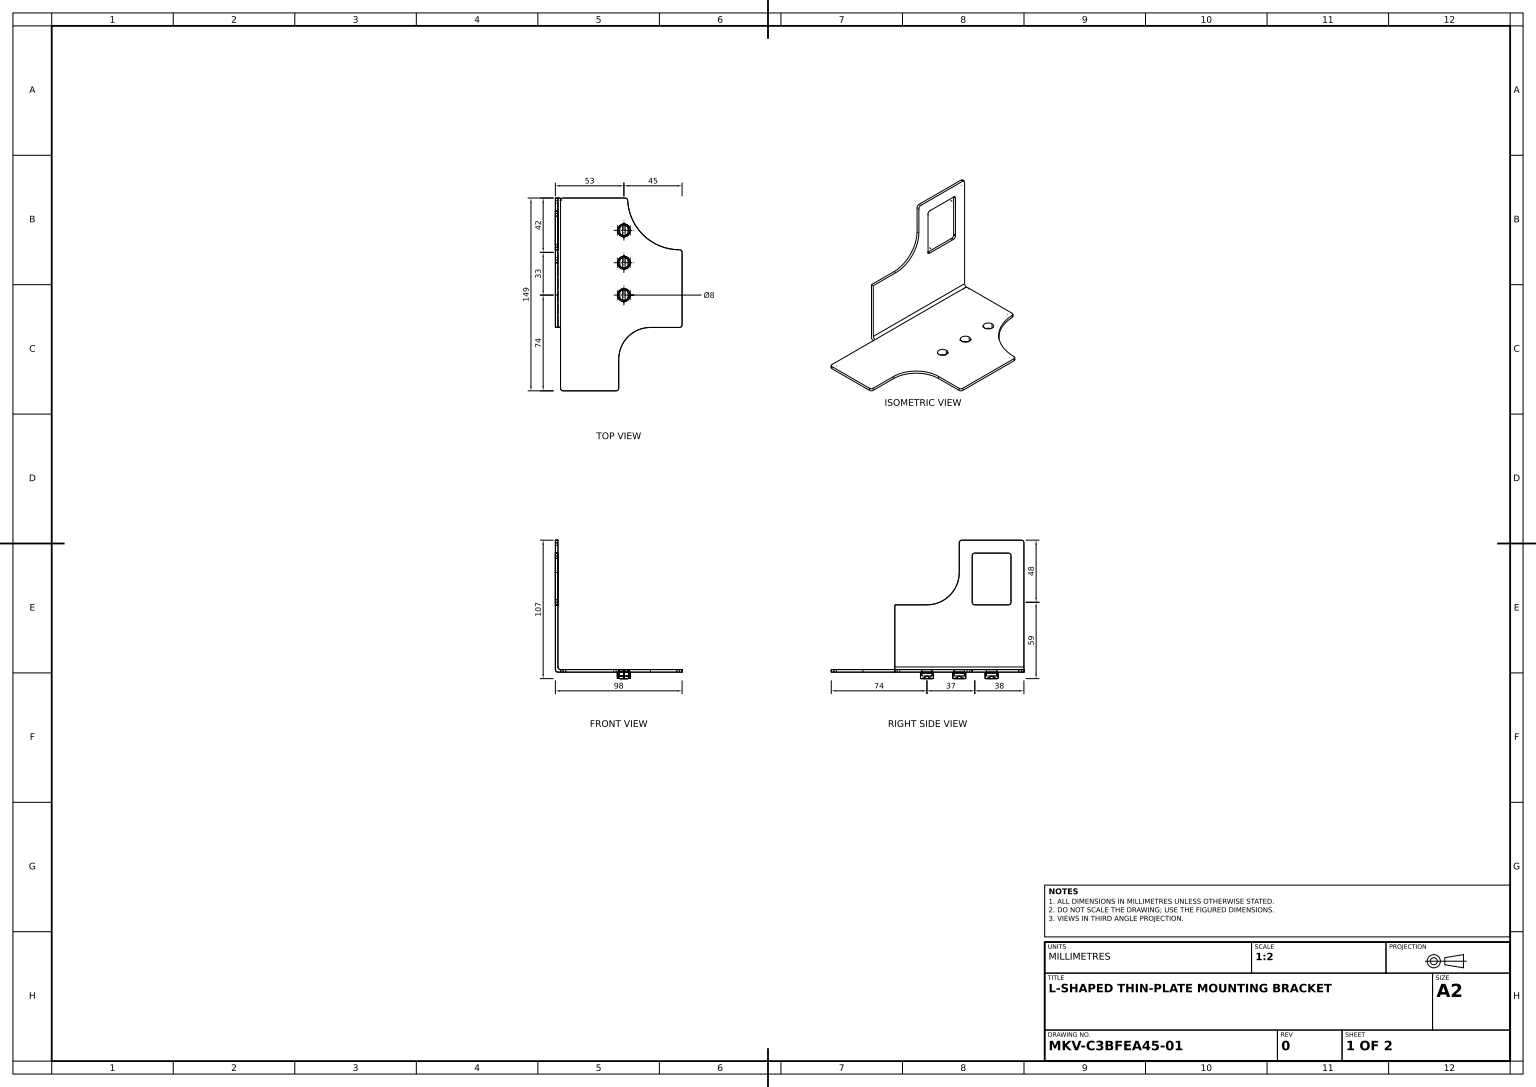
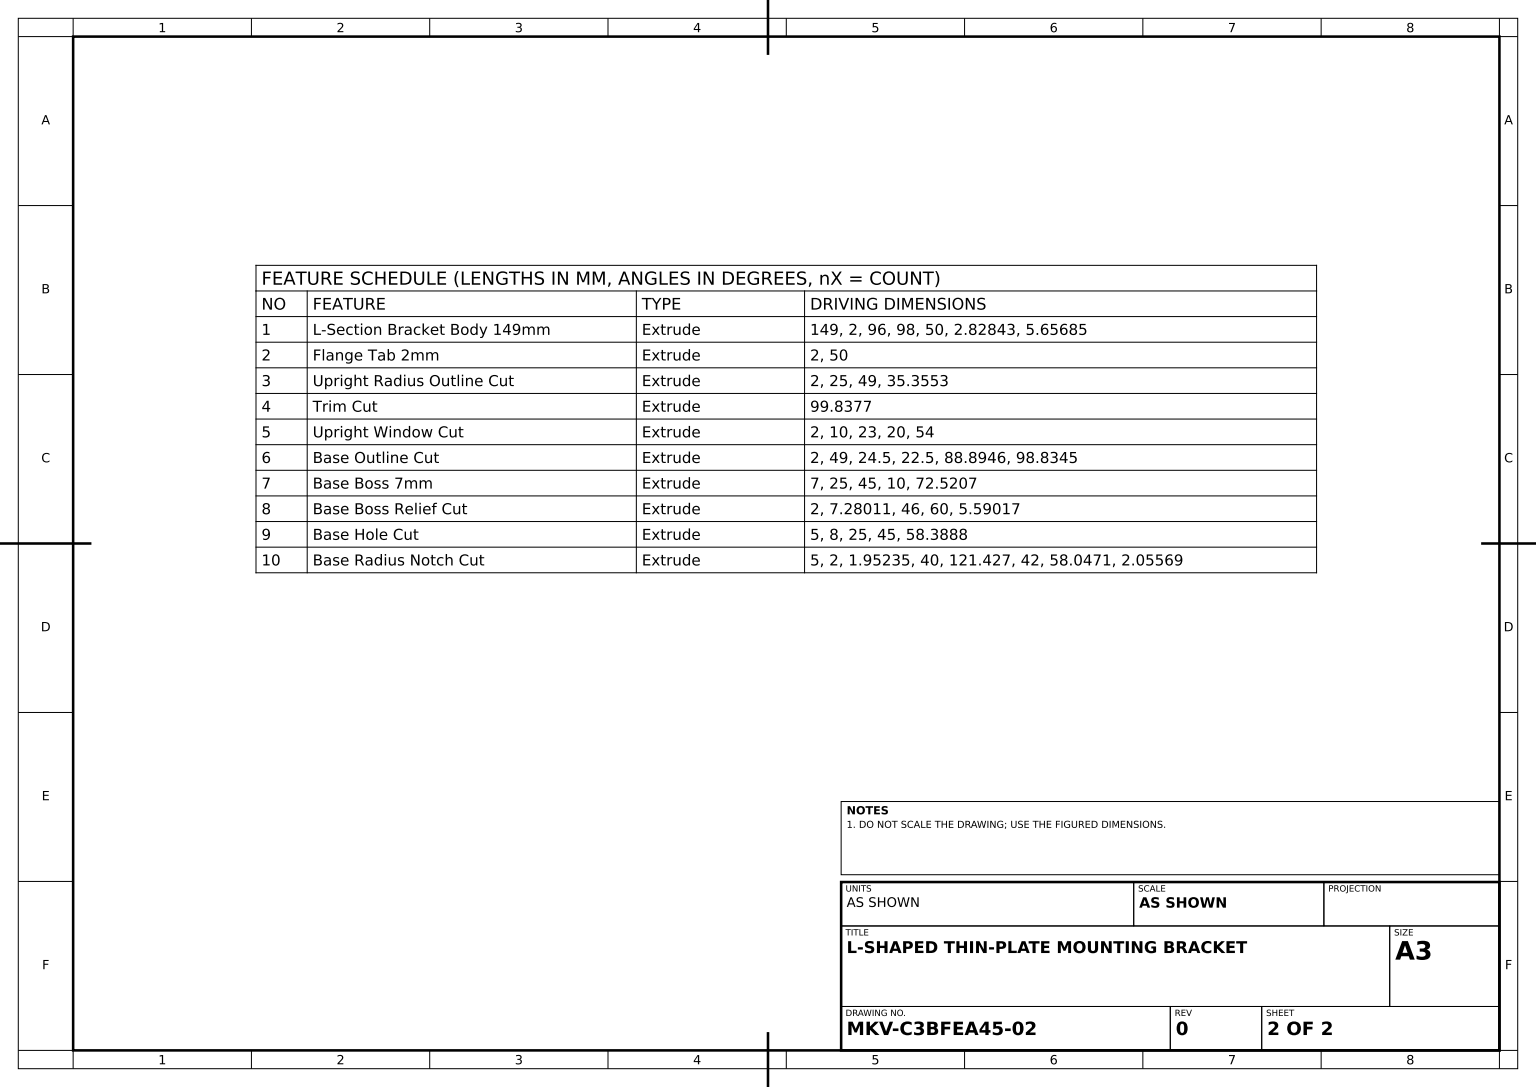
SolidWorks part; units mm, degrees
material "Plain Carbon Steel"
ref_plane "Front Plane" through (0, 0, 0) normal (0, 0, 1) x (1, 0, 0)
ref_plane "Top Plane" through (0, 0, 0) normal (0, 1, 0) x (1, 0, 0)
ref_plane "Right Plane" through (0, 0, 0) normal (1, 0, 0) x (0, 0, -1)
sketch "L-Section Profile Sketch" plane through (0, 0, 0) normal (0, 0, 1) x (1, 0, 0)
  line L0 (2, 0) -> (98, 0)
  line L4 (0, 2) -> (0, 52)
  line L5 (0, 52) -> (2, 52)
  line L6 (2, 52) -> (2, 4)
  line L7 (4, 2) -> (98, 2)
  line L8 (98, 2) -> (98, 0)
  arc A0 (2, 4) -> (4, 2) centre (4, 4) ccw
  arc A2 (0, 2) -> (2, 0) centre (2, 2) ccw
  dimension "D2" = 2
  dimension "D1" = 2
  dimension "D3" = 96
  dimension "D4" = 98
  dimension "D5" = 50
  dimension "D6" = 2
  dimension "D7" = 2
  dimension "D8" = 2.8284
  dimension "D9" = 5.6569
extrude "L-Section Bracket Body 149mm" add sketch "L-Section Profile Sketch" along normal mid plane 149
sketch "Flange Tab Sketch" plane through (2, 0, 0) normal (1, 0, 0) x (0, 0, -1)
  line L0 (74.5, 52) -> (74.5, 102)
  line L1 (74.5, 102) -> (-74.5, 102)
  line L2 (-74.5, 102) -> (-74.5, 52)
  line L3 (-74.5, 52) -> (74.5, 52)
  line L5 (-74.5, 52) -> (74.5, 52) construction
  dimension "D1" = 50
extrude "Flange Tab 2mm" add sketch "Flange Tab Sketch" against normal blind 2
sketch "Upright Radius Outline Sketch" plane through (2, 0, 0) normal (1, 0, 0) x (0, 0, -1)
  line L0 (24.5, 102) -> (-74.5, 102)
  line L1 (-74.5, 102) -> (-74.5, 4)
  line L2 (74.5, 102) -> (-74.5, 102) construction
  line L3 (-74.5, 4) -> (-25.5, 4)
  line L4 (-74.5, 4) -> (74.5, 4) construction
  line L5 (-25.5, 4) -> (-25.5, 52)
  line L6 (-25.5, 52) -> (-0.5, 52)
  line L7 (24.5, 77) -> (24.5, 102)
  arc A0 (-0.5, 52) -> (24.5, 77) centre (-0.5, 77) ccw
  dimension "D1" = 25
  dimension "D2" = 25
  dimension "D3" = 49
  dimension "D4" = 35.3553
extrude "Upright Radius Outline Cut" cut sketch "Upright Radius Outline Sketch" against normal blind 2
sketch "Trim Cut Sketch" plane through (0, 2, 0) normal (0, 1, 0) x (1, 0, 0)
  line L0 (0, -25.3377) -> (4, -25.3377)
  line L1 (4, -74.5) -> (4, 74.5) construction
  line L2 (4, -25.3377) -> (4, -74.5)
  line L3 (4, -74.5) -> (0, -74.5)
  line L4 (0, -74.5) -> (0, -25.3377)
  line L5 (98, 74.5) -> (4, 74.5) construction
  dimension "D1" = 99.8377
extrude "Trim Cut" cut sketch "Trim Cut Sketch" along normal through all both and the other way through all
sketch "Upright Window Sketch" plane through (2, 0, 0) normal (1, 0, 0) x (0, 0, -1)
  line L0 (74.5, 102) -> (72.5, 102)
  line L2 (-25.3377, 4) -> (74.5, 4) construction
  line L3 (24.5811, 4) -> (74.5, 4)
  line L4 (74.5, 100) -> (74.5, 102)
  line L5 (49.5, 102) -> (49.5, 52) construction
  line L6 (49.5, 102) -> (49.5, 92) construction
  line L7 (24.5, 102) -> (24.5, 100)
  line L8 (36.5, 92) -> (62.5, 92)
  line L9 (34.5, 90) -> (34.5, 54)
  line L10 (36.5, 52) -> (62.5, 52)
  line L11 (64.5, 90) -> (64.5, 54)
  line L12 (34.5, 102) -> (61.482, 102) construction
  line L13 (74.5, 102) -> (24.5, 102) construction
  line L14 (74.5, 102) -> (74.5, 100)
  line L15 (26.5, 102) -> (24.5, 102)
  line L16 (49.5, 72) -> (59.9531, 72) construction
  arc A1 (26.5, 102) -> (24.5, 100) centre (26.5, 100) ccw
  arc A2 (72.5, 102) -> (74.5, 100) centre (72.5, 100) cw
  arc A3 (36.5, 92) -> (34.5, 90) centre (36.5, 90) ccw
  arc A4 (62.5, 92) -> (64.5, 90) centre (62.5, 90) cw
  arc A5 (62.5, 52) -> (64.5, 54) centre (62.5, 54) ccw
  arc A6 (36.5, 52) -> (34.5, 54) centre (36.5, 54) cw
  point P13 (49.5, 72)
  line M11 (74.5, 4) -> (74.5, 102)
  line M12 (74.5, 102) -> (24.5, 102)
  line M13 (24.5, 102) -> (24.5, 77)
  dimension "D1" = 10
  dimension "D5" = 2
  dimension "D2" = 2
  dimension "D3" = 54
  dimension "D4" = 10
  dimension "D6" = 23
  dimension "D8" = 20
extrude "Upright Window Cut" cut sketch "Upright Window Sketch" against normal blind 2 contours A1 M12 M13 | A2 M12 M11 | A6 L10 A5 L11 A4 L8 A3 L9
sketch "Base Outline Sketch" plane through (0, 2, 0) normal (0, 1, 0) x (1, 0, 0)
  line L0 (4, 74.5) -> (4, 72.5)
  line L1 (4, -74.5) -> (6, -74.5)
  line L2 (98, -74.5) -> (98, -23.5)
  line L3 (6, 74.5) -> (4, 74.5)
  line L4 (0, 0) -> (98, 0) construction
  line L5 (98, -74.5) -> (49, -74.5) construction
  line L6 (49, -72.5) -> (49, -50) construction
  line L7 (73.5, -25.5) -> (96, -25.5) construction
  line L8 (49, -50) -> (49, -72.5)
  line L9 (73.5, -25.5) -> (96, -25.5)
  line L10 (47, -74.5) -> (98, -74.5)
  line L11 (4, -72.5) -> (4, -74.5)
  line L12 (4, 72.5) -> (4, 74.5)
  line L13 (4, 74.5) -> (6, 74.5)
  arc A0 (4, -72.5) -> (6, -74.5) centre (6, -72.5) ccw
  arc A2 (73.5, -25.5) -> (49, -50) centre (73.5, -50) ccw
  arc A4 (47, -74.5) -> (49, -72.5) centre (47, -72.5) ccw
  arc A5 (96, -25.5) -> (98, -23.5) centre (96, -23.5) ccw
  arc A6 (4, 72.5) -> (6, 74.5) centre (6, 72.5) cw
  line M8 (98, 74.5) -> (4, 74.5)
  line M9 (4, 74.5) -> (4, -25.3377)
  line M10 (4, -25.3377) -> (4, -74.5)
  line M11 (4, -74.5) -> (98, -74.5)
  line M12 (98, -74.5) -> (98, 74.5)
  dimension "D1" = 49
  dimension "D2" = 24.5
  dimension "D3" = 2
  dimension "D4" = 2
  dimension "D8" = 2
  dimension "D5" = 22.5
  dimension "D6" = 88.8946
  dimension "D7" = 98.8345
extrude "Base Outline Cut" cut sketch "Base Outline Sketch" against normal blind 2 contours A6 M9 M8 | A5 L9 A2 L8 A4 M11 M12 | A0 M10 M11
sketch "Base Boss Sketch" plane through (0, 2, 0) normal (0, 1, 0) x (1, 0, 0)
  line L0 (98, 74.5) -> (98, 49.5) construction
  line L1 (98, -23.5) -> (98, 74.5) construction
  line L2 (98, 49.5) -> (98, 24.5) construction
  line L3 (98, 24.5) -> (53, 24.5) construction
  circle A0 centre (53, 24.5) radius 5
  circle A1 centre (53, 49.5) radius 5
  circle A2 centre (53, -0.5) radius 5
  dimension "D4" = 10
  dimension "D5" = 10
  dimension "D1" = 25
  dimension "D2" = 25
  dimension "D3" = 45
  dimension "D6" = 25
  dimension "D7" = 72.5207
extrude "Base Boss 7mm" add sketch "Base Boss Sketch" against normal blind 7
sketch "Base Boss Relief Sketch" plane through (0, 0, 0) normal (0, 0, 1) x (1, 0, 0)
  line L1 (47, 0) -> (49, 0) construction
  line L4 (58, -5) -> (56, -5)
  line L5 (58, -3) -> (58, -5)
  line L7 (46, 0) -> (48, 0)
  line L9 (46, 0) -> (48, 0)
  line L10 (46, 0) -> (48, 0)
  line L11 (48, -2) -> (48, 0)
  line L12 (48, 0) -> (58, 0)
  line L13 (49, 0) -> (73.5, 0) construction
  line L14 (48, 0) -> (58, 0) construction
  line L15 (58, 0) -> (58, -2)
  line L16 (53, 0) -> (53, -5) construction
  line L17 (58, -2.5) -> (48, -2.5) construction
  line L18 (48, 0) -> (48, -5) construction
  line L19 (58, -2) -> (58, 0)
  line L20 (60, 0) -> (58, 0)
  line L21 (48, -3) -> (48, -5)
  line L22 (48, -5) -> (50, -5)
  arc A0 (48, -2) -> (46, 0) centre (46, -2) ccw
  arc A2 (58, -2) -> (60, 0) centre (60, -2) cw
  arc A3 (48, -3) -> (50, -5) centre (50, -3) ccw
  arc A4 (58, -3) -> (56, -5) centre (56, -3) cw
  dimension "D1" = 2
  dimension "D4" = 2
  dimension "D5" = 60
  dimension "D2" = 7.2801
  dimension "D3" = 46
  dimension "D6" = 5.5902
extrude "Base Boss Relief Cut" cut sketch "Base Boss Relief Sketch" against normal through all both and the other way through all contours A3 L21 L22 | L5 A4 L4
sketch "Base Hole Sketch" plane through (0, 2, 0) normal (0, 1, 0) x (1, 0, 0)
  line L0 (98, 74.5) -> (98, 49.5) construction
  line L1 (98, -23.5) -> (98, 74.5) construction
  line L2 (98, 49.5) -> (98, 24.5) construction
  line L3 (98, 24.5) -> (53, 24.5) construction
  line L4 (98, 49.5) -> (53, 49.5) construction
  circle A0 centre (53, 24.5) radius 4
  circle A2 centre (53, 49.5) radius 4
  circle A3 centre (53, -0.5) radius 4
  dimension "D1" = 45
  dimension "D2" = 8
  dimension "D5" = 8
  dimension "D3" = 25
  dimension "D4" = 25
  dimension "D6" = 58.3888
extrude "Base Hole Cut" cut sketch "Base Hole Sketch" against normal blind 5
sketch "Base Radius Notch Sketch" plane through (0, 2, 0) normal (0, 1, 0) x (1, 0, 0)
  line L0 (55.8872, 74.5) -> (53.9348, 74.5)
  line L1 (98, 74.5) -> (6, 74.5) construction
  line L2 (98, -23.5) -> (98, 74.5) construction
  line L3 (55.8872, 74.5) -> (98, 74.5)
  line L4 (98, 74.5) -> (98, 34.5558)
  line L5 (98, 34.5558) -> (98, 32.5002)
  arc A0 (55.9325, 72.5952) -> (95.9946, 34.5001) centre (95.8872, 74.5) ccw
  arc A2 (55.9325, 72.5952) -> (53.9348, 74.5) centre (53.9348, 72.5) ccw
  arc A3 (98, 32.5002) -> (95.9946, 34.5001) centre (96, 32.5002) ccw
  dimension "D1" = 2
  dimension "D3" = 40
  dimension "D2" = 1.9524
  dimension "D4" = 121.4273
  dimension "D5" = 42
  dimension "D6" = 58.0471
  dimension "D7" = 2.0557
extrude "Base Radius Notch Cut" cut sketch "Base Radius Notch Sketch" against normal blind 5
